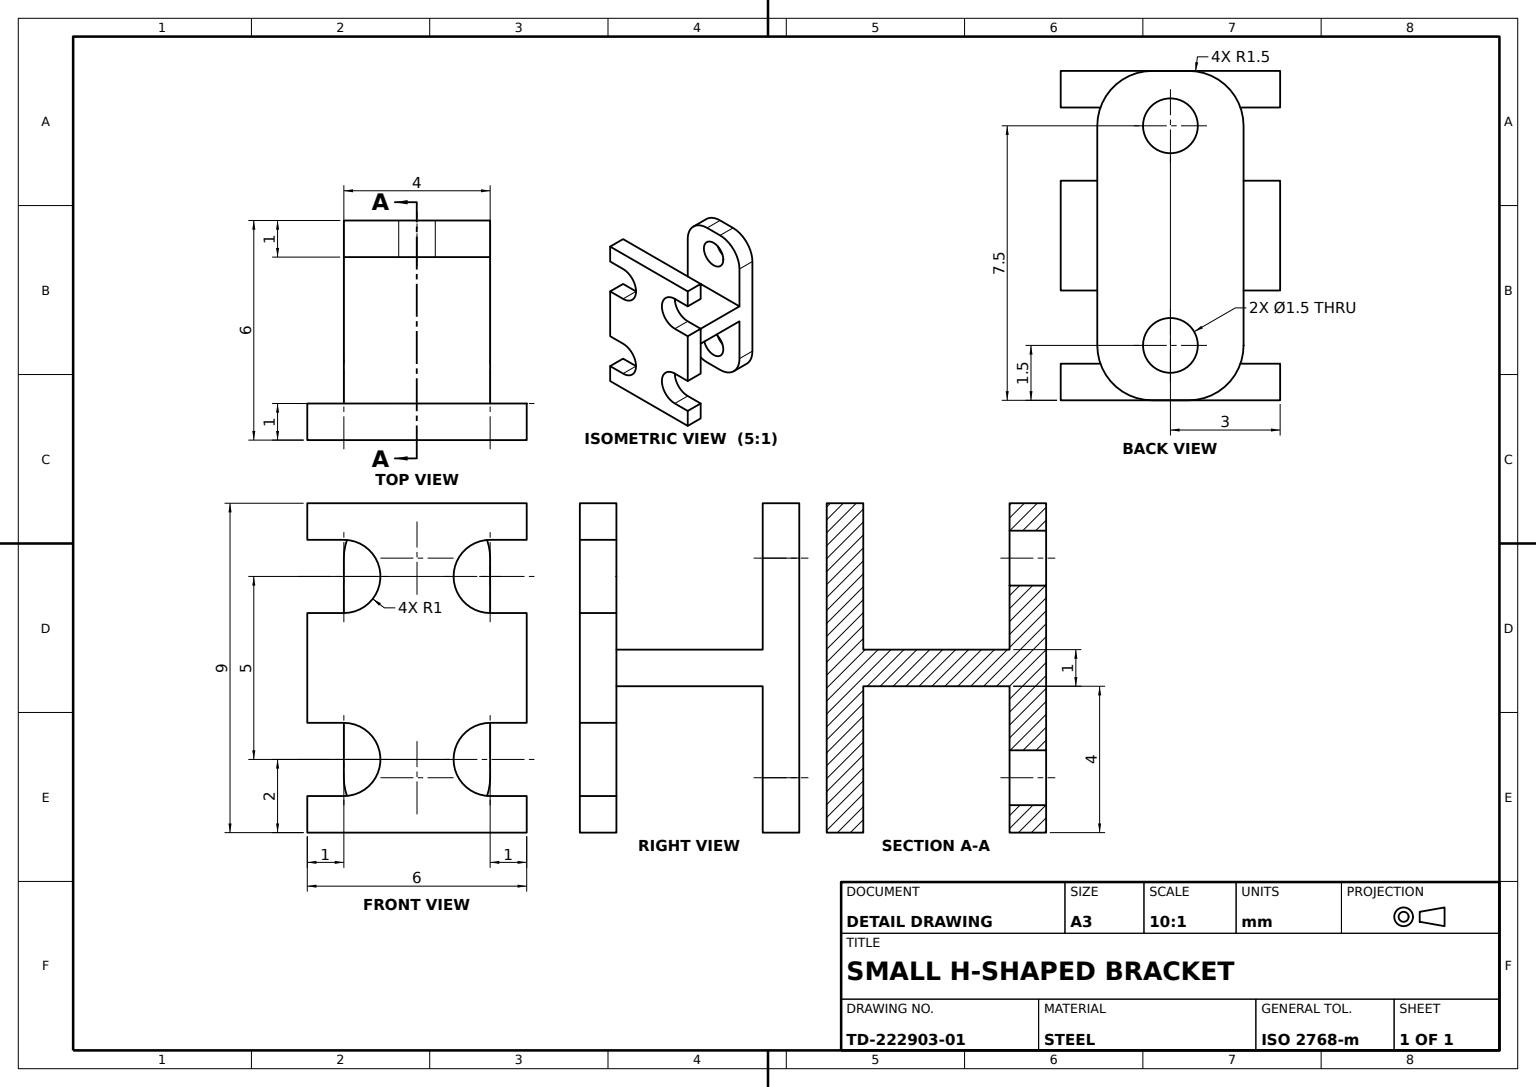
SolidWorks part; units mm, degrees
material "Plain Carbon Steel"
ref_plane "Front Plane" through (0, 0, 0) normal (0, 0, 1) x (1, 0, 0)
ref_plane "Top Plane" through (0, 0, 0) normal (0, 1, 0) x (1, 0, 0)
ref_plane "Right Plane" through (0, 0, 0) normal (1, 0, 0) x (0, 0, -1)
sketch "Base Plate Sketch" plane through (0, 0, 0) normal (0, 0, 1) x (1, 0, 0)
  line L0 (0, 0) -> (6, 0)
  line L1 (6, 0) -> (6, 1)
  line L2 (6, 3) -> (5, 3)
  line L3 (6, 1) -> (5, 1)
  line L4 (0, 9) -> (0, 8)
  line L5 (6, 3) -> (6, 6)
  line L6 (6, 8) -> (5, 8)
  line L7 (6, 6) -> (5, 6)
  line L8 (0, 8) -> (1, 8)
  line L9 (6, 8) -> (6, 9)
  line L10 (6, 9) -> (0, 9)
  line L12 (1, 6) -> (0, 6)
  line L13 (0, 6) -> (0, 3)
  line L14 (0, 3) -> (1, 3)
  line L16 (1, 1) -> (0, 1)
  line L17 (0, 1) -> (0, 0)
  arc A0 (5, 8) -> (5, 6) centre (5, 7) ccw
  arc A1 (5, 3) -> (5, 1) centre (5, 2) ccw
  arc A2 (1, 8) -> (1, 6) centre (1, 7) cw
  arc A3 (1, 3) -> (1, 1) centre (1, 2) cw
  dimension "D1" = 6
  dimension "D2" = 1
  dimension "D4" = 2
  dimension "D8" = 9
  dimension "D9" = 1
  dimension "D3" = 3
  dimension "D5" = 1
  dimension "D6" = 6
  dimension "D7" = 3
  dimension "D10" = 1
  dimension "D11" = 5
  dimension "D12" = 6
  dimension "D13" = 5
  dimension "D14" = 1
extrude "Base Plate" add sketch "Base Plate Sketch" along normal blind 1
sketch "Standoff Web Sketch" plane through (0, 0, 0) normal (0, 0, -1) x (-1, 0, 0)
  line L0 (0, 9) -> (0, 8) construction
  line L1 (-5, 5) -> (-1, 5)
  line L2 (-5, 5) -> (-5, 4)
  line L3 (-5, 4) -> (-1, 4)
  line L4 (-1, 5) -> (-1, 4)
  line L5 (-5, 5) -> (-1, 4) construction
  line L6 (-5, 4) -> (-1, 5) construction
  line L7 (-6, 9) -> (0, 9) construction
  point P0 (-3, 4.5)
  dimension "D1" = 1
  dimension "D2" = 3
  dimension "D3" = 4
  dimension "D4" = 4.5
extrude "Standoff Web 4mm" add sketch "Standoff Web Sketch" along normal blind 4
sketch "Fork Lug Sketch" plane through (0, 0, -4) normal (0, 0, -1) x (-1, 0, 0)
  line L0 (0, 0) -> (-6, 0) construction
  line L1 (-5, 9) -> (-1, 9)
  line L2 (-5, 9) -> (-5, 0)
  line L3 (-5, 0) -> (-1, 0)
  line L4 (-1, 9) -> (-1, 0)
  line L5 (-5, 9) -> (-1, 0) construction
  line L6 (-5, 0) -> (-1, 9) construction
  line L7 (-1, 4) -> (-1, 5) construction
  line L8 (-1, 5) -> (-5, 5) construction
  point P0 (-3, 4.5)
  dimension "D1" = 2
  dimension "D2" = 4
  dimension "D3" = 4
extrude "Fork Lug" add sketch "Fork Lug Sketch" along normal blind 1
fillet "Lug End Fillets R1.5" radius 1.5 4 edges at (1, 0, -4.5) (5, 0, -4.5) (1, 9, -4.5) (5, 9, -4.5)
sketch "Lug Pin Holes Sketch" plane through (0, 0, -5) normal (0, 0, -1) x (-1, 0, 0)
  line L0 (-1, 1.5) -> (-1, 7.5) construction
  line L1 (-3.5, 0) -> (-2.5, 0) construction
  circle A0 centre (-3, 7.5) radius 0.75
  circle A1 centre (-3, 1.5) radius 0.7496
  dimension "D1" = 1.5
  dimension "D2" = 1.4991
  dimension "D3" = 2
  dimension "D4" = 1.5
  dimension "D5" = 7.5
extrude "Lug Pin Holes" cut sketch "Lug Pin Holes Sketch" against normal blind 1
